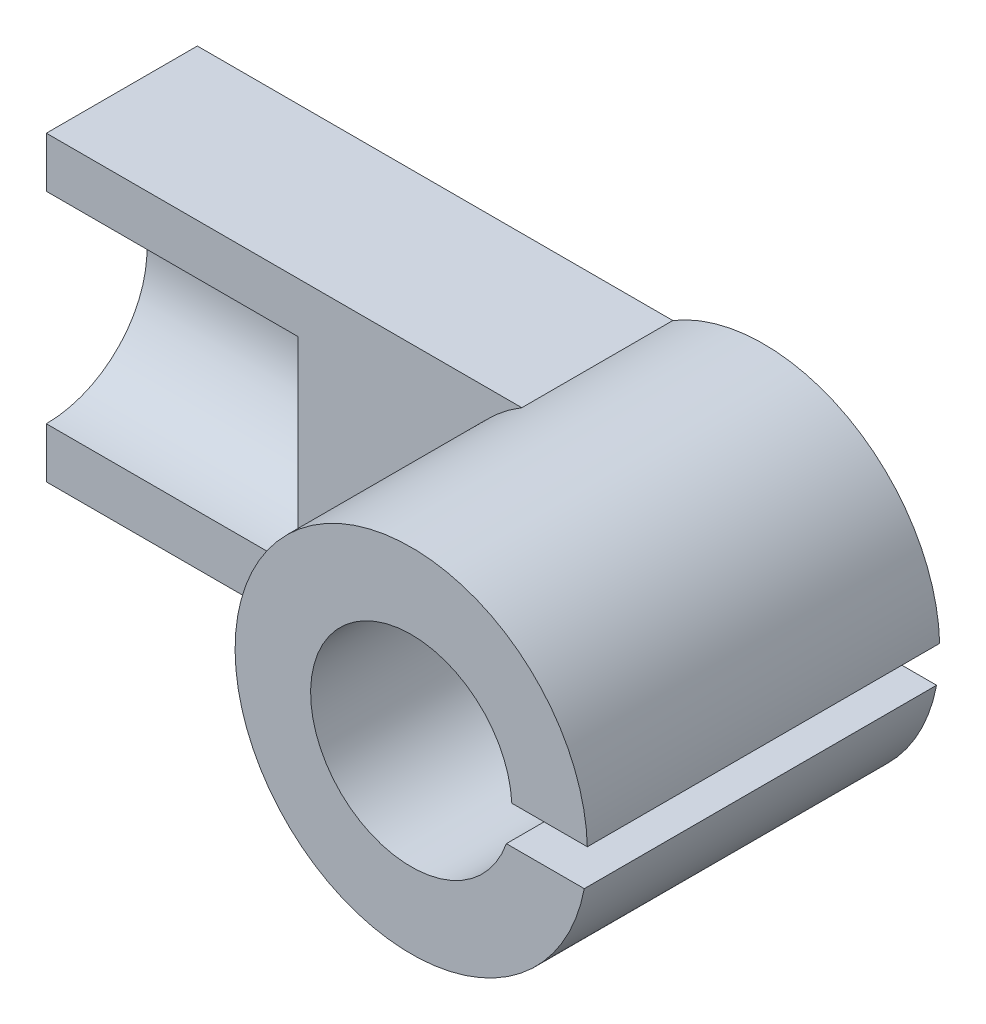
ISO-10303-21;
HEADER;
FILE_DESCRIPTION(('STEP AP214'),'2;1');
FILE_NAME('part.step','',(''),(''),'','','');
FILE_SCHEMA(('AUTOMOTIVE_DESIGN { 1 0 10303 214 1 1 1 1 }'));
ENDSEC;
DATA;
#1=APPLICATION_CONTEXT('core data for automotive mechanical design processes');
#2=APPLICATION_PROTOCOL_DEFINITION('international standard','automotive_design',2000,#1);
#3=PRODUCT_CONTEXT('',#1,'mechanical');
#4=PRODUCT('Part','Part','',(#3));
#5=PRODUCT_RELATED_PRODUCT_CATEGORY('part','',(#4));
#6=PRODUCT_DEFINITION_FORMATION('','',#4);
#7=PRODUCT_DEFINITION_CONTEXT('part definition',#1,'design');
#8=PRODUCT_DEFINITION('design','',#6,#7);
#9=PRODUCT_DEFINITION_SHAPE('','',#8);
#10=(LENGTH_UNIT() NAMED_UNIT(*) SI_UNIT(.MILLI.,.METRE.));
#11=(NAMED_UNIT(*) PLANE_ANGLE_UNIT() SI_UNIT($,.RADIAN.));
#12=(NAMED_UNIT(*) SI_UNIT($,.STERADIAN.) SOLID_ANGLE_UNIT());
#13=UNCERTAINTY_MEASURE_WITH_UNIT(LENGTH_MEASURE(1.E-05),#10,'distance_accuracy_value','');
#14=(GEOMETRIC_REPRESENTATION_CONTEXT(3) GLOBAL_UNCERTAINTY_ASSIGNED_CONTEXT((#13)) GLOBAL_UNIT_ASSIGNED_CONTEXT((#10,
#11,#12)) REPRESENTATION_CONTEXT('',''));
#15=CARTESIAN_POINT('',(0.,0.,0.));
#16=DIRECTION('',(0.,0.,1.));
#17=DIRECTION('',(1.,0.,0.));
#18=AXIS2_PLACEMENT_3D('',#15,#16,#17);
#19=CARTESIAN_POINT('',(45.,24.,12.));
#20=DIRECTION('',(-1.,0.,0.));
#21=DIRECTION('',(0.,0.,1.));
#22=AXIS2_PLACEMENT_3D('',#19,#20,#21);
#23=PLANE('',#22);
#24=DIRECTION('',(0.,0.,-1.));
#25=VECTOR('',#24,1.);
#26=CARTESIAN_POINT('',(45.,16.,44.));
#27=LINE('',#26,#25);
#28=CARTESIAN_POINT('',(45.,16.,12.));
#29=VERTEX_POINT('',#28);
#30=CARTESIAN_POINT('',(45.,16.,-12.));
#31=VERTEX_POINT('',#30);
#32=EDGE_CURVE('E154',#29,#31,#27,.T.);
#33=ORIENTED_EDGE('',*,*,#32,.F.);
#34=DIRECTION('',(0.,1.,0.));
#35=VECTOR('',#34,1.);
#36=CARTESIAN_POINT('',(45.,24.,12.));
#37=LINE('',#36,#35);
#38=CARTESIAN_POINT('',(45.,-16.,12.));
#39=VERTEX_POINT('',#38);
#40=EDGE_CURVE('E180',#39,#29,#37,.T.);
#41=ORIENTED_EDGE('',*,*,#40,.F.);
#42=DIRECTION('',(0.,0.,-1.));
#43=VECTOR('',#42,1.);
#44=CARTESIAN_POINT('',(45.,-16.,44.));
#45=LINE('',#44,#43);
#46=CARTESIAN_POINT('',(45.,-16.,-12.));
#47=VERTEX_POINT('',#46);
#48=EDGE_CURVE('E148',#47,#39,#45,.F.);
#49=ORIENTED_EDGE('',*,*,#48,.F.);
#50=DIRECTION('',(0.,1.,0.));
#51=VECTOR('',#50,1.);
#52=CARTESIAN_POINT('',(45.,24.,-12.));
#53=LINE('',#52,#51);
#54=EDGE_CURVE('E174',#47,#31,#53,.T.);
#55=ORIENTED_EDGE('',*,*,#54,.T.);
#56=EDGE_LOOP('',(#33,#41,#49,#55));
#57=FACE_BOUND('',#56,.T.);
#58=ADVANCED_FACE('F39',(#57),#23,.F.);
#59=CARTESIAN_POINT('',(0.,0.,12.));
#60=DIRECTION('',(0.,0.,1.));
#61=DIRECTION('',(1.,0.,0.));
#62=AXIS2_PLACEMENT_3D('',#59,#60,#61);
#63=PLANE('',#62);
#64=ORIENTED_EDGE('',*,*,#40,.T.);
#65=CARTESIAN_POINT('',(45.,0.,12.));
#66=DIRECTION('',(0.,0.,1.));
#67=DIRECTION('',(1.,0.,0.));
#68=AXIS2_PLACEMENT_3D('',#65,#66,#67);
#69=CIRCLE('',#68,16.);
#70=EDGE_CURVE('E142',#29,#39,#69,.T.);
#71=ORIENTED_EDGE('',*,*,#70,.T.);
#72=EDGE_LOOP('',(#64,#71));
#73=FACE_BOUND('',#72,.T.);
#74=ADVANCED_FACE('F253',(#73),#63,.T.);
#75=CARTESIAN_POINT('',(-45.,24.,12.));
#76=DIRECTION('',(0.,-1.,0.));
#77=DIRECTION('',(0.,0.,-1.));
#78=AXIS2_PLACEMENT_3D('',#75,#76,#77);
#79=PLANE('',#78);
#80=DIRECTION('',(-1.,0.,0.));
#81=VECTOR('',#80,1.);
#82=CARTESIAN_POINT('',(-45.,24.,12.));
#83=LINE('',#82,#81);
#84=CARTESIAN_POINT('',(30.577794898144,24.,12.));
#85=VERTEX_POINT('',#84);
#86=CARTESIAN_POINT('',(-45.,24.,12.));
#87=VERTEX_POINT('',#86);
#88=EDGE_CURVE('E179',#85,#87,#83,.T.);
#89=ORIENTED_EDGE('',*,*,#88,.F.);
#90=DIRECTION('',(0.,0.,-1.));
#91=VECTOR('',#90,1.);
#92=CARTESIAN_POINT('',(30.577794898144,24.,44.));
#93=LINE('',#92,#91);
#94=CARTESIAN_POINT('',(30.577794898144,24.,-12.));
#95=VERTEX_POINT('',#94);
#96=EDGE_CURVE('E165',#85,#95,#93,.T.);
#97=ORIENTED_EDGE('',*,*,#96,.T.);
#98=DIRECTION('',(-1.,0.,0.));
#99=VECTOR('',#98,1.);
#100=CARTESIAN_POINT('',(-45.,24.,-12.));
#101=LINE('',#100,#99);
#102=CARTESIAN_POINT('',(-45.,24.,-12.));
#103=VERTEX_POINT('',#102);
#104=EDGE_CURVE('E192',#95,#103,#101,.T.);
#105=ORIENTED_EDGE('',*,*,#104,.T.);
#106=DIRECTION('',(0.,0.,-1.));
#107=VECTOR('',#106,1.);
#108=CARTESIAN_POINT('',(-45.,24.,12.));
#109=LINE('',#108,#107);
#110=EDGE_CURVE('E133',#87,#103,#109,.T.);
#111=ORIENTED_EDGE('',*,*,#110,.F.);
#112=EDGE_LOOP('',(#89,#97,#105,#111));
#113=FACE_BOUND('',#112,.T.);
#114=ADVANCED_FACE('F226',(#113),#79,.F.);
#115=CARTESIAN_POINT('',(-45.,24.,12.));
#116=DIRECTION('',(1.,0.,0.));
#117=DIRECTION('',(0.,1.,0.));
#118=AXIS2_PLACEMENT_3D('',#115,#116,#117);
#119=PLANE('',#118);
#120=DIRECTION('',(0.,-1.,0.));
#121=VECTOR('',#120,1.);
#122=CARTESIAN_POINT('',(-45.,24.,12.));
#123=LINE('',#122,#121);
#124=CARTESIAN_POINT('',(-45.,-16.,12.));
#125=VERTEX_POINT('',#124);
#126=CARTESIAN_POINT('',(-45.,-24.,12.));
#127=VERTEX_POINT('',#126);
#128=EDGE_CURVE('E181',#125,#127,#123,.T.);
#129=ORIENTED_EDGE('',*,*,#128,.F.);
#130=CARTESIAN_POINT('',(-45.,0.,12.));
#131=DIRECTION('',(-1.,0.,0.));
#132=DIRECTION('',(0.,-1.,0.));
#133=AXIS2_PLACEMENT_3D('',#130,#131,#132);
#134=CIRCLE('',#133,16.);
#135=CARTESIAN_POINT('',(-45.,16.,12.));
#136=VERTEX_POINT('',#135);
#137=EDGE_CURVE('E164',#136,#125,#134,.T.);
#138=ORIENTED_EDGE('',*,*,#137,.F.);
#139=EDGE_CURVE('E184',#87,#136,#123,.T.);
#140=ORIENTED_EDGE('',*,*,#139,.F.);
#141=ORIENTED_EDGE('',*,*,#110,.T.);
#142=DIRECTION('',(0.,-1.,0.));
#143=VECTOR('',#142,1.);
#144=CARTESIAN_POINT('',(-45.,24.,-12.));
#145=LINE('',#144,#143);
#146=CARTESIAN_POINT('',(-45.,-24.,-12.));
#147=VERTEX_POINT('',#146);
#148=EDGE_CURVE('E194',#103,#147,#145,.T.);
#149=ORIENTED_EDGE('',*,*,#148,.T.);
#150=DIRECTION('',(0.,0.,-1.));
#151=VECTOR('',#150,1.);
#152=CARTESIAN_POINT('',(-45.,-24.,12.));
#153=LINE('',#152,#151);
#154=EDGE_CURVE('E189',#127,#147,#153,.T.);
#155=ORIENTED_EDGE('',*,*,#154,.F.);
#156=EDGE_LOOP('',(#129,#138,#140,#141,#149,#155));
#157=FACE_BOUND('',#156,.T.);
#158=ADVANCED_FACE('F210',(#157),#119,.F.);
#159=CARTESIAN_POINT('',(-45.,-24.,12.));
#160=DIRECTION('',(0.,1.,0.));
#161=DIRECTION('',(0.,0.,1.));
#162=AXIS2_PLACEMENT_3D('',#159,#160,#161);
#163=PLANE('',#162);
#164=DIRECTION('',(1.,0.,0.));
#165=VECTOR('',#164,1.);
#166=CARTESIAN_POINT('',(-45.,-24.,-12.));
#167=LINE('',#166,#165);
#168=CARTESIAN_POINT('',(30.577794898144,-24.,-12.));
#169=VERTEX_POINT('',#168);
#170=EDGE_CURVE('E182',#147,#169,#167,.T.);
#171=ORIENTED_EDGE('',*,*,#170,.T.);
#172=DIRECTION('',(0.,0.,-1.));
#173=VECTOR('',#172,1.);
#174=CARTESIAN_POINT('',(30.577794898144,-24.,44.));
#175=LINE('',#174,#173);
#176=CARTESIAN_POINT('',(30.577794898144,-24.,12.));
#177=VERTEX_POINT('',#176);
#178=EDGE_CURVE('E157',#169,#177,#175,.F.);
#179=ORIENTED_EDGE('',*,*,#178,.T.);
#180=DIRECTION('',(1.,0.,0.));
#181=VECTOR('',#180,1.);
#182=CARTESIAN_POINT('',(-45.,-24.,12.));
#183=LINE('',#182,#181);
#184=EDGE_CURVE('E190',#127,#177,#183,.T.);
#185=ORIENTED_EDGE('',*,*,#184,.F.);
#186=ORIENTED_EDGE('',*,*,#154,.T.);
#187=EDGE_LOOP('',(#171,#179,#185,#186));
#188=FACE_BOUND('',#187,.T.);
#189=ADVANCED_FACE('F220',(#188),#163,.F.);
#190=CARTESIAN_POINT('',(45.,0.,12.));
#191=DIRECTION('',(0.,0.,1.));
#192=DIRECTION('',(1.,0.,0.));
#193=AXIS2_PLACEMENT_3D('',#190,#191,#192);
#194=CIRCLE('',#193,28.);
#195=EDGE_CURVE('E160',#85,#177,#194,.T.);
#196=ORIENTED_EDGE('',*,*,#195,.F.);
#197=ORIENTED_EDGE('',*,*,#88,.T.);
#198=ORIENTED_EDGE('',*,*,#139,.T.);
#199=DIRECTION('',(-1.,0.,0.));
#200=VECTOR('',#199,1.);
#201=CARTESIAN_POINT('',(-5.,16.,12.));
#202=LINE('',#201,#200);
#203=CARTESIAN_POINT('',(-5.,16.,12.));
#204=VERTEX_POINT('',#203);
#205=EDGE_CURVE('E168',#204,#136,#202,.T.);
#206=ORIENTED_EDGE('',*,*,#205,.F.);
#207=DIRECTION('',(0.,1.,0.));
#208=VECTOR('',#207,1.);
#209=CARTESIAN_POINT('',(-5.,0.,12.));
#210=LINE('',#209,#208);
#211=CARTESIAN_POINT('',(-4.99999999999999,-16.,12.));
#212=VERTEX_POINT('',#211);
#213=EDGE_CURVE('E167',#212,#204,#210,.T.);
#214=ORIENTED_EDGE('',*,*,#213,.F.);
#215=DIRECTION('',(-1.,0.,0.));
#216=VECTOR('',#215,1.);
#217=CARTESIAN_POINT('',(-5.,-16.,12.));
#218=LINE('',#217,#216);
#219=EDGE_CURVE('E175',#212,#125,#218,.T.);
#220=ORIENTED_EDGE('',*,*,#219,.T.);
#221=ORIENTED_EDGE('',*,*,#128,.T.);
#222=ORIENTED_EDGE('',*,*,#184,.T.);
#223=EDGE_LOOP('',(#196,#197,#198,#206,#214,#220,#221,#222));
#224=FACE_BOUND('',#223,.T.);
#225=ADVANCED_FACE('F222',(#224),#63,.T.);
#226=CARTESIAN_POINT('',(0.,0.,-12.));
#227=DIRECTION('',(0.,0.,1.));
#228=DIRECTION('',(1.,0.,0.));
#229=AXIS2_PLACEMENT_3D('',#226,#227,#228);
#230=PLANE('',#229);
#231=CARTESIAN_POINT('',(45.,0.,-12.));
#232=DIRECTION('',(0.,0.,-1.));
#233=DIRECTION('',(-1.,0.,0.));
#234=AXIS2_PLACEMENT_3D('',#231,#232,#233);
#235=CIRCLE('',#234,28.);
#236=CARTESIAN_POINT('',(72.9897190450315,0.758701377488086,-12.));
#237=VERTEX_POINT('',#236);
#238=EDGE_CURVE('E141',#95,#237,#235,.T.);
#239=ORIENTED_EDGE('',*,*,#238,.T.);
#240=DIRECTION('',(-1.,0.,0.));
#241=VECTOR('',#240,1.);
#242=CARTESIAN_POINT('',(57.6774885209343,0.758701377488086,-12.));
#243=LINE('',#242,#241);
#244=CARTESIAN_POINT('',(60.9820015085657,0.758701377488086,-12.));
#245=VERTEX_POINT('',#244);
#246=EDGE_CURVE('E231',#237,#245,#243,.T.);
#247=ORIENTED_EDGE('',*,*,#246,.T.);
#248=CARTESIAN_POINT('',(45.,0.,-12.));
#249=DIRECTION('',(0.,0.,-1.));
#250=DIRECTION('',(-1.,0.,0.));
#251=AXIS2_PLACEMENT_3D('',#248,#249,#250);
#252=CIRCLE('',#251,16.);
#253=EDGE_CURVE('E151',#31,#245,#252,.T.);
#254=ORIENTED_EDGE('',*,*,#253,.F.);
#255=ORIENTED_EDGE('',*,*,#54,.F.);
#256=CARTESIAN_POINT('',(60.1171686750415,-5.24129862251191,-12.));
#257=VERTEX_POINT('',#256);
#258=EDGE_CURVE('E243',#257,#47,#252,.T.);
#259=ORIENTED_EDGE('',*,*,#258,.F.);
#260=DIRECTION('',(1.,0.,0.));
#261=VECTOR('',#260,1.);
#262=CARTESIAN_POINT('',(76.6267989254012,-5.24129862251191,-12.));
#263=LINE('',#262,#261);
#264=CARTESIAN_POINT('',(72.5050684192869,-5.24129862251191,-12.));
#265=VERTEX_POINT('',#264);
#266=EDGE_CURVE('E233',#257,#265,#263,.T.);
#267=ORIENTED_EDGE('',*,*,#266,.T.);
#268=EDGE_CURVE('E137',#265,#169,#235,.T.);
#269=ORIENTED_EDGE('',*,*,#268,.T.);
#270=ORIENTED_EDGE('',*,*,#170,.F.);
#271=ORIENTED_EDGE('',*,*,#148,.F.);
#272=ORIENTED_EDGE('',*,*,#104,.F.);
#273=EDGE_LOOP('',(#239,#247,#254,#255,#259,#267,#269,#270,#271,#272));
#274=FACE_BOUND('',#273,.T.);
#275=ADVANCED_FACE('F214',(#274),#230,.F.);
#276=CARTESIAN_POINT('',(-5.,0.,12.));
#277=DIRECTION('',(-1.,0.,0.));
#278=DIRECTION('',(0.,-1.,0.));
#279=AXIS2_PLACEMENT_3D('',#276,#277,#278);
#280=CYLINDRICAL_SURFACE('',#279,16.);
#281=ORIENTED_EDGE('',*,*,#137,.T.);
#282=ORIENTED_EDGE('',*,*,#219,.F.);
#283=CARTESIAN_POINT('',(-5.,0.,12.));
#284=DIRECTION('',(-1.,0.,0.));
#285=DIRECTION('',(0.,-1.,0.));
#286=AXIS2_PLACEMENT_3D('',#283,#284,#285);
#287=CIRCLE('',#286,16.);
#288=EDGE_CURVE('E169',#204,#212,#287,.T.);
#289=ORIENTED_EDGE('',*,*,#288,.F.);
#290=ORIENTED_EDGE('',*,*,#205,.T.);
#291=EDGE_LOOP('',(#281,#282,#289,#290));
#292=FACE_BOUND('',#291,.T.);
#293=ADVANCED_FACE('F230',(#292),#280,.F.);
#294=CARTESIAN_POINT('',(-5.,0.,0.));
#295=DIRECTION('',(-1.,0.,0.));
#296=DIRECTION('',(0.,-1.,0.));
#297=AXIS2_PLACEMENT_3D('',#294,#295,#296);
#298=PLANE('',#297);
#299=ORIENTED_EDGE('',*,*,#213,.T.);
#300=ORIENTED_EDGE('',*,*,#288,.T.);
#301=EDGE_LOOP('',(#299,#300));
#302=FACE_BOUND('',#301,.T.);
#303=ADVANCED_FACE('F278',(#302),#298,.T.);
#304=CARTESIAN_POINT('',(45.,0.,44.));
#305=DIRECTION('',(0.,0.,-1.));
#306=DIRECTION('',(-1.,0.,0.));
#307=AXIS2_PLACEMENT_3D('',#304,#305,#306);
#308=CYLINDRICAL_SURFACE('',#307,28.);
#309=DIRECTION('',(0.,0.,-1.));
#310=VECTOR('',#309,1.);
#311=CARTESIAN_POINT('',(72.9897190450315,0.758701377488086,44.));
#312=LINE('',#311,#310);
#313=CARTESIAN_POINT('',(72.9897190450315,0.758701377488086,44.));
#314=VERTEX_POINT('',#313);
#315=EDGE_CURVE('E52',#237,#314,#312,.F.);
#316=ORIENTED_EDGE('',*,*,#315,.F.);
#317=ORIENTED_EDGE('',*,*,#238,.F.);
#318=ORIENTED_EDGE('',*,*,#96,.F.);
#319=ORIENTED_EDGE('',*,*,#195,.T.);
#320=ORIENTED_EDGE('',*,*,#178,.F.);
#321=ORIENTED_EDGE('',*,*,#268,.F.);
#322=DIRECTION('',(0.,0.,-1.));
#323=VECTOR('',#322,1.);
#324=CARTESIAN_POINT('',(72.5050684192869,-5.24129862251191,44.));
#325=LINE('',#324,#323);
#326=CARTESIAN_POINT('',(72.5050684192869,-5.24129862251191,44.));
#327=VERTEX_POINT('',#326);
#328=EDGE_CURVE('E124',#327,#265,#325,.T.);
#329=ORIENTED_EDGE('',*,*,#328,.F.);
#330=CARTESIAN_POINT('',(45.,0.,44.));
#331=DIRECTION('',(0.,0.,-1.));
#332=DIRECTION('',(-1.,0.,0.));
#333=AXIS2_PLACEMENT_3D('',#330,#331,#332);
#334=CIRCLE('',#333,28.);
#335=EDGE_CURVE('E136',#327,#314,#334,.T.);
#336=ORIENTED_EDGE('',*,*,#335,.T.);
#337=EDGE_LOOP('',(#316,#317,#318,#319,#320,#321,#329,#336));
#338=FACE_BOUND('',#337,.T.);
#339=ADVANCED_FACE('F134',(#338),#308,.T.);
#340=CARTESIAN_POINT('',(45.,0.,44.));
#341=DIRECTION('',(0.,0.,-1.));
#342=DIRECTION('',(-1.,0.,0.));
#343=AXIS2_PLACEMENT_3D('',#340,#341,#342);
#344=CYLINDRICAL_SURFACE('',#343,16.);
#345=ORIENTED_EDGE('',*,*,#253,.T.);
#346=DIRECTION('',(0.,0.,-1.));
#347=VECTOR('',#346,1.);
#348=CARTESIAN_POINT('',(60.9820015085657,0.758701377488086,44.));
#349=LINE('',#348,#347);
#350=CARTESIAN_POINT('',(60.9820015085657,0.758701377488086,44.));
#351=VERTEX_POINT('',#350);
#352=EDGE_CURVE('E138',#245,#351,#349,.F.);
#353=ORIENTED_EDGE('',*,*,#352,.T.);
#354=CARTESIAN_POINT('',(45.,0.,44.));
#355=DIRECTION('',(0.,0.,-1.));
#356=DIRECTION('',(-1.,0.,0.));
#357=AXIS2_PLACEMENT_3D('',#354,#355,#356);
#358=CIRCLE('',#357,16.);
#359=CARTESIAN_POINT('',(60.1171686750415,-5.24129862251191,44.));
#360=VERTEX_POINT('',#359);
#361=EDGE_CURVE('E238',#360,#351,#358,.T.);
#362=ORIENTED_EDGE('',*,*,#361,.F.);
#363=DIRECTION('',(0.,0.,-1.));
#364=VECTOR('',#363,1.);
#365=CARTESIAN_POINT('',(60.1171686750415,-5.24129862251191,44.));
#366=LINE('',#365,#364);
#367=EDGE_CURVE('E58',#360,#257,#366,.T.);
#368=ORIENTED_EDGE('',*,*,#367,.T.);
#369=ORIENTED_EDGE('',*,*,#258,.T.);
#370=ORIENTED_EDGE('',*,*,#48,.T.);
#371=ORIENTED_EDGE('',*,*,#70,.F.);
#372=ORIENTED_EDGE('',*,*,#32,.T.);
#373=EDGE_LOOP('',(#345,#353,#362,#368,#369,#370,#371,#372));
#374=FACE_BOUND('',#373,.T.);
#375=ADVANCED_FACE('F236',(#374),#344,.F.);
#376=CARTESIAN_POINT('',(45.,0.,44.));
#377=DIRECTION('',(0.,0.,-1.));
#378=DIRECTION('',(-1.,0.,0.));
#379=AXIS2_PLACEMENT_3D('',#376,#377,#378);
#380=PLANE('',#379);
#381=ORIENTED_EDGE('',*,*,#361,.T.);
#382=DIRECTION('',(1.,0.,0.));
#383=VECTOR('',#382,1.);
#384=CARTESIAN_POINT('',(45.,0.758701377488086,44.));
#385=LINE('',#384,#383);
#386=EDGE_CURVE('E11',#351,#314,#385,.T.);
#387=ORIENTED_EDGE('',*,*,#386,.T.);
#388=ORIENTED_EDGE('',*,*,#335,.F.);
#389=DIRECTION('',(-1.,0.,0.));
#390=VECTOR('',#389,1.);
#391=CARTESIAN_POINT('',(45.,-5.24129862251191,44.));
#392=LINE('',#391,#390);
#393=EDGE_CURVE('E46',#327,#360,#392,.T.);
#394=ORIENTED_EDGE('',*,*,#393,.T.);
#395=EDGE_LOOP('',(#381,#387,#388,#394));
#396=FACE_BOUND('',#395,.T.);
#397=ADVANCED_FACE('F143',(#396),#380,.F.);
#398=CARTESIAN_POINT('',(76.6267989254012,-5.24129862251191,-12.));
#399=DIRECTION('',(0.,-1.,0.));
#400=DIRECTION('',(0.,0.,-1.));
#401=AXIS2_PLACEMENT_3D('',#398,#399,#400);
#402=PLANE('',#401);
#403=ORIENTED_EDGE('',*,*,#328,.T.);
#404=ORIENTED_EDGE('',*,*,#266,.F.);
#405=ORIENTED_EDGE('',*,*,#367,.F.);
#406=ORIENTED_EDGE('',*,*,#393,.F.);
#407=EDGE_LOOP('',(#403,#404,#405,#406));
#408=FACE_BOUND('',#407,.T.);
#409=ADVANCED_FACE('F123',(#408),#402,.F.);
#410=CARTESIAN_POINT('',(57.6774885209343,0.758701377488086,-12.));
#411=DIRECTION('',(0.,1.,0.));
#412=DIRECTION('',(0.,0.,1.));
#413=AXIS2_PLACEMENT_3D('',#410,#411,#412);
#414=PLANE('',#413);
#415=ORIENTED_EDGE('',*,*,#315,.T.);
#416=ORIENTED_EDGE('',*,*,#386,.F.);
#417=ORIENTED_EDGE('',*,*,#352,.F.);
#418=ORIENTED_EDGE('',*,*,#246,.F.);
#419=EDGE_LOOP('',(#415,#416,#417,#418));
#420=FACE_BOUND('',#419,.T.);
#421=ADVANCED_FACE('F336',(#420),#414,.F.);
#422=CLOSED_SHELL('',(#58,#74,#114,#158,#189,#225,#275,#293,#303,#339,#375,#397,#409,#421));
#423=MANIFOLD_SOLID_BREP('B2',#422);
#424=ADVANCED_BREP_SHAPE_REPRESENTATION('',(#18,#423),#14);
#425=SHAPE_DEFINITION_REPRESENTATION(#9,#424);
ENDSEC;
END-ISO-10303-21;
